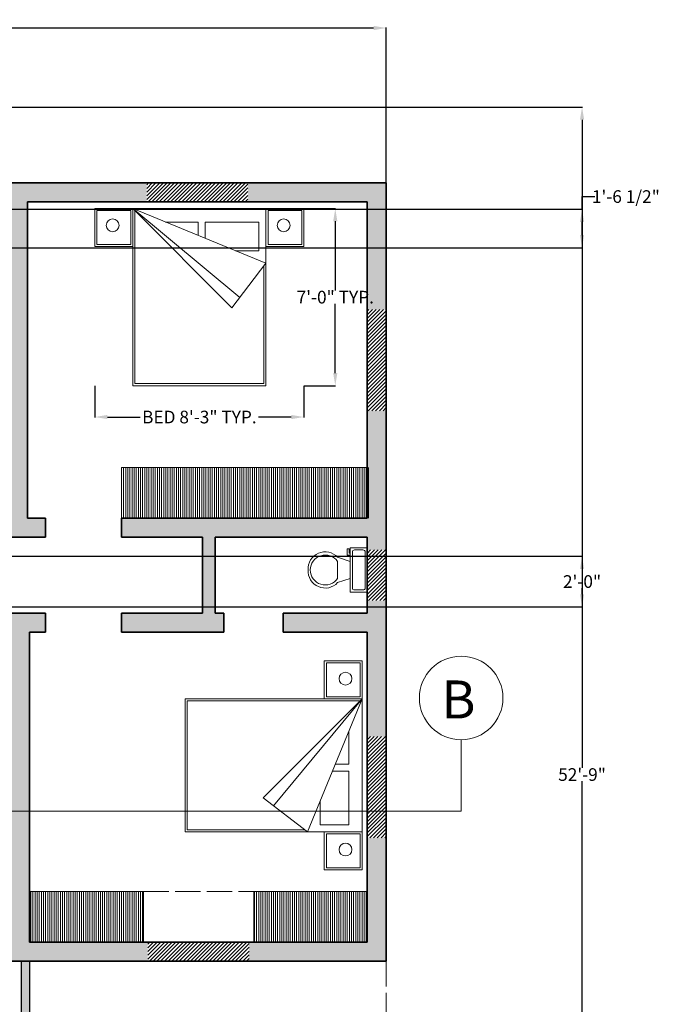
# Model space of a CAD drawing. Units: inches. Extents: x 1966 to 4198, y 2607 to 3884.
# Tile 7 of 8: x 3172 to 3474, y 3411 to 3878. Entities that reach past the tile are written whole.
import ezdxf

# ---------------------------------------------------------------- set-up
doc = ezdxf.new("R2010")
doc.units = ezdxf.units.IN
doc.header["$MEASUREMENT"] = 0
doc.linetypes.add('ACAD_ISO02W100', pattern=[15, 12, -3])
for name, color, linetype, lineweight in [('A-ANNO-SYMB', 90, 'Continuous', 18), ('A-FLOR', 7, 'Continuous', 25), ('A-FLOR-CASE', 163, 'Continuous', 18), ('A-FLOR-CASE-HIDN', 163, 'ACAD_ISO02W100', 13), ('A-FLOR-CASE-PATT', 163, 'Continuous', 13), ('A-FLOR-FIXT', 163, 'Continuous', 18), ('A-GLAZ-PATT', 14, 'Continuous', 13), ('A-WALL', 7, 'Continuous', 35), ('A-WALL-PATT', 252, 'Continuous', 13), ('C-PRKG', 10, 'ACAD_ISO02W100', 18), ('dimension', 90, 'Continuous', 18), ('furniture', 163, 'Continuous', 18)]:
    doc.layers.add(name, color=color, linetype=linetype, lineweight=lineweight)
doc.styles.get("Standard").update_dxf_attribs({"font": 'arial.ttf'})
doc.dimstyles.get("Standard").update_dxf_attribs({"dimtxt": 6, "dimasz": 6, "dimexe": 0.18, "dimexo": 0.0625, "dimgap": 0.09, "dimtad": 0, "dimtih": 1, "dimtoh": 1, "dimdec": 1, "dimzin": 0, "dimdsep": 46, "dimlunit": 3, "dimtxsty": 'Standard', "dimcen": 0.09, "dimadec": 0, "dimazin": 0, "dimtfac": 1, "dimtdec": 1, "dimtofl": 0, "dimtmove": 0, "dimatfit": 3, "dimfxl": 1, "dimtolj": 1, "dimtzin": 0, "dimarcsym": 0})

# ---------------------------------------------------------------- blocks, each defined once
blk = doc.blocks.new('*U14')
for p, q in [((9.5, -6), (9.5, -2)), ((-10, -8.5), (-8, -8.5)), ((-10, -9.5), (-10, -8.5)), ((-8, -8.5), (-8, -8)), ((-7, -8), (-7, -9.5)), ((-4, -8), (-6, -14)), ((4, -8), (6, -14)), ((-7, -9.5), (-10, -9.5)), ((4, -14), (-4, -14))]:
    blk.add_line(p, q)
blk.add_lwpolyline([(10.5, -8), (10.5, 0), (-10.5, 0), (-10.5, -8)], close=True)
for points in [[(-9.5, -2), (-9.5, -6)], [(8.5, -1), (-8.5, -1)], [(-8.5, -7), (8.5, -7)]]:
    blk.add_lwpolyline(points)
for centre, radius, start, end in [((-8.625, -1.875), 0.8839, 81.8699, 188.1301), ((8.625, -1.875), 0.8839, 351.8699, 98.1301), ((-8.625, -6.125), 0.8839, 171.869898, 278.1301), ((8.625, -6.125), 0.8839, 261.8699, 8.1301), ((-0.4772, -19.9188), 8.0953, 133.01722, 273.38), ((0.0374, -19.8731), 7.127, 124.50543, 269.7), ((-0.0373, -19.8731), 7.127, 270.3, 55.4946), ((0.4773, -19.9188), 8.0953, 266.62, 46.9828)]:
    blk.add_arc(centre, radius, start, end)
blk = doc.blocks.new('BED')
at = {"layer": 'furniture'}
for p, q in [((3238.51, 3777.61), (3301.62, 3751.64)), ((3285.43, 3730.55), (3238.51, 3777.61)), ((3238.51, 3777.61), (3289.22, 3735.48)), ((3301.62, 3751.64), (3285.43, 3730.55))]:
    blk.add_line(p, q, dxfattribs=at)
for points in [[(3220.51, 3759.61), (3238.51, 3759.61), (3238.51, 3777.61), (3220.51, 3777.61)], [(3238.51, 3693.61), (3301.62, 3693.61), (3301.62, 3777.61), (3238.51, 3777.61)], [(3301.62, 3759.61), (3319.62, 3759.61), (3319.62, 3777.61), (3301.62, 3777.61)], [(3221.51, 3760.61), (3237.51, 3760.61), (3237.51, 3776.61), (3221.51, 3776.61)], [(3302.62, 3760.61), (3318.62, 3760.61), (3318.62, 3776.61), (3302.62, 3776.61)]]:
    blk.add_lwpolyline(points, close=True, dxfattribs=at)
for points in [[(3239.51, 3776.61), (3239.51, 3694.61), (3300.62, 3694.61), (3300.62, 3750.34)], [(3254.03, 3771.22), (3269.45, 3771.22), (3269.45, 3764.88)], [(3272.78, 3763.51), (3272.78, 3771.22), (3298.23, 3771.22), (3298.23, 3757.59), (3287.16, 3757.59)]]:
    blk.add_lwpolyline(points, dxfattribs=at)
for centre in [(3228.96, 3769.64), (3310.01, 3769.64)]:
    blk.add_circle(centre, 3.03, dxfattribs=at)
blk = doc.blocks.new('PORCH-PARAPET-PLAN')
for p, q in [((0, 86), (0, 0)), ((4, 86), (4, 4)), ((181.42, 86), (181.42, 4)), ((185.42, 86), (185.42, 0)), ((0, 0), (23.64, 0)), ((4, 4), (23.64, 4)), ((23.64, 4), (23.64, 0)), ((83.64, 4), (83.64, 0)), ((83.64, 4), (181.42, 4)), ((83.64, 0), (185.42, 0))]:
    blk.add_line(p, q)
blk = doc.blocks.new('*D51')
at = {"layer": 'Defpoints', "color": 0, "transparency": 16777216}
for p in [(3207.34, 3704.37), (3306.44, 3704.37), (3306.44, 3689.51)]:
    blk.add_point(p, dxfattribs=at)
at = {"layer": 'dimension', "color": 0, "lineweight": -2, "transparency": 16777216}
for p, q in [((3207.34, 3704.31), (3207.34, 3689.33)), ((3306.44, 3704.31), (3306.44, 3689.33)), ((3213.34, 3689.51), (3228.87, 3689.51)), ((3300.44, 3689.51), (3284.92, 3689.51))]:
    blk.add_line(p, q, dxfattribs=at)
at = {"layer": 'dimension', "color": 0, "transparency": 16777216}
for points in [[(3213.34, 3690.51), (3213.34, 3688.51), (3207.34, 3689.51)], [(3300.44, 3690.51), (3300.44, 3688.51), (3306.44, 3689.51)]]:
    blk.add_solid(points, dxfattribs=at)
at = {"layer": 'dimension', "color": 0, "transparency": 16777216, "insert": (3256.89, 3689.51), "char_height": 6, "attachment_point": 5}
blk.add_mtext('\\A1;BED 8\'-3" TYP.', dxfattribs=at)
blk = doc.blocks.new('*D52')
at = {"layer": 'Defpoints', "color": 0, "transparency": 16777216}
for p in [(3306.44, 3788.37), (3321.31, 3788.37), (3306.44, 3704.37)]:
    blk.add_point(p, dxfattribs=at)
at = {"layer": 'dimension', "color": 0, "lineweight": -2, "transparency": 16777216}
for p, q in [((3306.51, 3788.37), (3321.49, 3788.37)), ((3321.31, 3782.37), (3321.31, 3749.53)), ((3321.31, 3710.37), (3321.31, 3743.22)), ((3306.51, 3704.37), (3321.49, 3704.37))]:
    blk.add_line(p, q, dxfattribs=at)
at = {"layer": 'dimension', "color": 0, "transparency": 16777216}
for points in [[(3320.31, 3782.37), (3322.31, 3782.37), (3321.31, 3788.37)], [(3320.31, 3710.37), (3322.31, 3710.37), (3321.31, 3704.37)]]:
    blk.add_solid(points, dxfattribs=at)
at = {"layer": 'dimension', "color": 0, "transparency": 16777216, "insert": (3321.31, 3746.37), "char_height": 6, "attachment_point": 5}
blk.add_mtext('\\A1;7\'-0" TYP.', dxfattribs=at)
blk = doc.blocks.new('*D87')
at = {"layer": 'Defpoints', "color": 0, "transparency": 16777216}
for p in [(3345.44, 3874), (2880.44, 3800.5), (3345.44, 3800.5)]:
    blk.add_point(p, dxfattribs=at)
at = {"layer": 'dimension', "color": 0, "lineweight": -2, "transparency": 16777216}
for p, q in [((2880.44, 3800.57), (2880.44, 3874.18)), ((2886.44, 3874), (3102.55, 3874)), ((3339.44, 3874), (3123.33, 3874)), ((3345.44, 3800.57), (3345.44, 3874.18))]:
    blk.add_line(p, q, dxfattribs=at)
at = {"layer": 'dimension', "color": 0, "transparency": 16777216}
for points in [[(2886.44, 3875), (2886.44, 3873), (2880.44, 3874)], [(3339.44, 3875), (3339.44, 3873), (3345.44, 3874)]]:
    blk.add_solid(points, dxfattribs=at)
at = {"layer": 'dimension', "color": 0, "transparency": 16777216, "insert": (3112.94, 3874), "char_height": 6, "attachment_point": 5}
blk.add_mtext('\\A1;38\'-9"', dxfattribs=at)
blk = doc.blocks.new('*D88')
at = {"layer": 'Defpoints', "color": 0, "transparency": 16777216}
for p in [(3058.44, 3836.5), (3345.44, 3203.44), (3438.28, 3203.44)]:
    blk.add_point(p, dxfattribs=at)
at = {"layer": 'dimension', "color": 0, "lineweight": -2, "transparency": 16777216}
for p, q in [((3058.5, 3836.5), (3438.46, 3836.5)), ((3438.28, 3830.5), (3438.28, 3523.13)), ((3438.28, 3209.44), (3438.28, 3516.82)), ((3345.5, 3203.44), (3438.46, 3203.44))]:
    blk.add_line(p, q, dxfattribs=at)
at = {"layer": 'dimension', "color": 0, "transparency": 16777216}
for points in [[(3437.28, 3830.5), (3439.28, 3830.5), (3438.28, 3836.5)], [(3437.28, 3209.44), (3439.28, 3209.44), (3438.28, 3203.44)]]:
    blk.add_solid(points, dxfattribs=at)
at = {"layer": 'dimension', "color": 0, "transparency": 16777216, "insert": (3438.28, 3519.97), "char_height": 6, "attachment_point": 5}
blk.add_mtext('\\A1;52\'-9"', dxfattribs=at)
blk = doc.blocks.new('*D93')
at = {"layer": 'Defpoints', "color": 0, "transparency": 16777216}
for p in [(2963.74, 3623.5), (3438.28, 3623.5), (2963.74, 3599.5)]:
    blk.add_point(p, dxfattribs=at)
at = {"layer": 'dimension', "color": 0, "lineweight": -2, "transparency": 16777216}
for p, q in [((2963.8, 3623.5), (3438.46, 3623.5)), ((3438.28, 3617.5), (3438.28, 3614.66)), ((3438.28, 3605.5), (3438.28, 3608.35)), ((2963.8, 3599.5), (3438.46, 3599.5))]:
    blk.add_line(p, q, dxfattribs=at)
at = {"layer": 'dimension', "color": 0, "transparency": 16777216}
for points in [[(3437.28, 3617.5), (3439.28, 3617.5), (3438.28, 3623.5)], [(3437.28, 3605.5), (3439.28, 3605.5), (3438.28, 3599.5)]]:
    blk.add_solid(points, dxfattribs=at)
at = {"layer": 'dimension', "color": 0, "transparency": 16777216, "insert": (3438.28, 3611.5), "char_height": 6, "attachment_point": 5}
blk.add_mtext('\\A1;2\'-0"', dxfattribs=at)
blk = doc.blocks.new('*D96')
at = {"layer": 'Defpoints', "color": 0, "transparency": 16777216}
for p in [(2967.99, 3788.06), (3438.28, 3788.06), (2967.99, 3769.8)]:
    blk.add_point(p, dxfattribs=at)
at = {"layer": 'dimension', "color": 0, "lineweight": -2, "transparency": 16777216}
for p, q in [((3438.28, 3788.06), (3438.28, 3794.06)), ((3438.28, 3794.06), (3444.28, 3794.06)), ((2968.06, 3788.06), (3438.46, 3788.06)), ((3438.28, 3775.8), (3438.28, 3782.06)), ((2968.06, 3769.8), (3438.46, 3769.8))]:
    blk.add_line(p, q, dxfattribs=at)
at = {"layer": 'dimension', "color": 0, "transparency": 16777216}
for points in [[(3437.28, 3782.06), (3439.28, 3782.06), (3438.28, 3788.06)], [(3437.28, 3775.8), (3439.28, 3775.8), (3438.28, 3769.8)]]:
    blk.add_solid(points, dxfattribs=at)
at = {"layer": 'dimension', "color": 0, "transparency": 16777216, "insert": (3459.06, 3794.06), "char_height": 6, "attachment_point": 5}
blk.add_mtext('\\A1;1\'-6 1/2"', dxfattribs=at)

msp = doc.modelspace()

# ---------------------------------------------------------------- hatches: boundary and pattern name
at = {"layer": 'A-FLOR-CASE-PATT'}
h = msp.add_hatch(dxfattribs=at)
h.set_pattern_fill('ANSI31', color=256, scale=8, angle=45, style=0)
h.paths.add_polyline_path([(3219.92, 3641.5), (3337.92, 3641.5), (3337.92, 3665.5), (3219.92, 3665.5)])
h = msp.add_hatch(dxfattribs=at)
h.set_pattern_fill('ANSI31', color=256, scale=8, angle=45, style=0)
h.paths.add_polyline_path([(3176.44, 3440.5), (3230.38, 3440.5), (3230.38, 3464.5), (3176.44, 3464.5)])
h = msp.add_hatch(dxfattribs=at)
h.set_pattern_fill('ANSI31', color=256, scale=8, angle=45, style=0)
h.paths.add_polyline_path([(3282.68, 3440.5), (3336.44, 3440.5), (3336.44, 3464.5), (3282.68, 3464.5)])
at = {"layer": 'A-GLAZ-PATT'}
h = msp.add_hatch(dxfattribs=at)
h.set_pattern_fill('ANSI31', color=256, scale=10)
h.set_pattern_definition([(45, (819.9656, 0), (-0.88388348, 0.88388348), [])])
h.paths.add_polyline_path([(2884.94, 3746.62), (2880.44, 3746.62), (2880.44, 3698.62), (2884.94, 3698.62)])
h.paths.add_polyline_path([(2889.44, 3746.62), (2884.94, 3746.62), (2884.94, 3698.62), (2889.44, 3698.62)])
h.paths.add_polyline_path([(2969.44, 3800.5), (2921.44, 3800.5), (2921.44, 3796), (2969.44, 3796)])
h.paths.add_polyline_path([(2969.44, 3796), (2921.44, 3796), (2921.44, 3791.5), (2969.44, 3791.5)])
h.paths.add_polyline_path([(3100.44, 3800.5), (3076.44, 3800.5), (3076.44, 3796), (3100.44, 3796)])
h.paths.add_polyline_path([(3100.44, 3796), (3076.44, 3796), (3076.44, 3791.5), (3100.44, 3791.5)])
h.paths.add_polyline_path([(3154.44, 3800.5), (3130.44, 3800.5), (3130.44, 3796), (3154.44, 3796)])
h.paths.add_polyline_path([(3154.44, 3796), (3130.44, 3796), (3130.44, 3791.5), (3154.44, 3791.5)])
h.paths.add_polyline_path([(3279.94, 3800.5), (3231.94, 3800.5), (3231.94, 3796), (3279.94, 3796)])
h.paths.add_polyline_path([(3279.94, 3796), (3231.94, 3796), (3231.94, 3791.5), (3279.94, 3791.5)])
h.paths.add_polyline_path([(3345.44, 3740.5), (3340.94, 3740.5), (3340.94, 3692.5), (3345.44, 3692.5)])
h.paths.add_polyline_path([(3340.94, 3740.5), (3336.44, 3740.5), (3336.44, 3692.5), (3340.94, 3692.5)])
h.paths.add_polyline_path([(3340.94, 3626.5), (3336.44, 3626.5), (3336.44, 3602.5), (3340.94, 3602.5)])
h.paths.add_polyline_path([(3345.44, 3626.5), (3340.94, 3626.5), (3340.94, 3602.5), (3345.44, 3602.5)])
h.paths.add_polyline_path([(3345.44, 3538), (3340.94, 3538), (3340.94, 3490), (3345.44, 3490)])
h.paths.add_polyline_path([(3340.94, 3538), (3336.44, 3538), (3336.44, 3490), (3340.94, 3490)])
h.paths.add_polyline_path([(3280.44, 3436), (3232.44, 3436), (3232.44, 3431.5), (3280.44, 3431.5)])
h.paths.add_polyline_path([(3280.44, 3440.5), (3232.44, 3440.5), (3232.44, 3436), (3280.44, 3436)])
at = {"layer": 'A-WALL-PATT'}
h = msp.add_hatch(color=256, dxfattribs=at)
h.dxf.hatch_style = 1
h.paths.add_polyline_path([(3010.44, 3599.5), (2889.44, 3599.5), (2889.44, 3698.62), (2880.44, 3698.62), (2880.44, 3590.5), (2880.44, 3539.5), (2889.44, 3539.5), (2889.44, 3590.5), (3010.44, 3590.5)])
h.paths.add_polyline_path([(2889.44, 3491.5), (2880.44, 3491.5), (2880.44, 3431.5), (2924.93, 3431.5), (2924.93, 3440.5), (2889.44, 3440.5)])
h.paths.add_polyline_path([(3008.43, 3440.5), (2972.93, 3440.5), (2972.93, 3431.5), (3008.43, 3431.5)])
h.paths.add_polyline_path([(2995.02, 3431.5), (2991.02, 3431.5), (2991.02, 3345.5), (3014.67, 3345.5), (3014.67, 3349.5), (2995.02, 3349.5)])
h.paths.add_polyline_path([(3232.44, 3440.5), (3176.44, 3440.5), (3176.44, 3587.5), (3183.92, 3587.5), (3183.92, 3591.41), (3183.92, 3596.5), (3167.44, 3596.5), (3167.44, 3440.5), (3092.44, 3440.5), (3092.44, 3590.5), (3083.44, 3590.5), (3083.44, 3440.5), (3056.43, 3440.5), (3056.43, 3438.68), (3056.43, 3431.5), (3092.44, 3431.5), (3232.44, 3431.5)])
h.paths.add_polyline_path([(3176.44, 3431.5), (3172.44, 3431.5), (3172.44, 3349.5), (3074.67, 3349.5), (3074.67, 3345.5), (3176.44, 3345.5)])
h.paths.add_polyline_path([(3345.44, 3490), (3336.44, 3490), (3336.44, 3440.5), (3280.44, 3440.5), (3280.44, 3431.5), (3345.44, 3431.5)])
h.paths.add_polyline_path([(3345.44, 3599.5), (3345.44, 3602.5), (3336.44, 3602.5), (3336.44, 3596.5), (3296.55, 3596.5), (3296.55, 3587.5), (3336.44, 3587.5), (3336.44, 3538), (3345.44, 3538)])
h.paths.add_polyline_path([(3264.44, 3632.5), (3336.44, 3632.5), (3336.44, 3626.5), (3345.44, 3626.5), (3345.44, 3692.5), (3336.44, 3692.5), (3336.44, 3641.5), (3219.92, 3641.5), (3219.92, 3632.5), (3258.44, 3632.5), (3258.44, 3596.5), (3219.95, 3596.5), (3219.95, 3591.41, -0.010779), (3219.92, 3589.86), (3219.92, 3587.5), (3268.55, 3587.5), (3268.55, 3591.7), (3268.55, 3596.5), (3264.44, 3596.5)])
h.paths.add_polyline_path([(3175.44, 3791.5), (3231.94, 3791.5), (3231.94, 3800.5), (3175.44, 3800.5), (3154.44, 3800.5), (3154.44, 3791.5), (3166.44, 3791.5), (3166.44, 3719.5), (3118.44, 3719.5), (3112.44, 3719.5), (3058.44, 3719.5), (3058.44, 3710.5), (3166.44, 3710.5), (3166.44, 3632.5), (3183.92, 3632.5), (3183.92, 3637.87), (3183.92, 3641.5), (3175.44, 3641.5)])
h.paths.add_polyline_path([(3345.44, 3800.5), (3279.94, 3800.5), (3279.94, 3791.5), (3336.44, 3791.5), (3336.44, 3740.5), (3345.44, 3740.5)])
h.paths.add_polyline_path([(3130.44, 3800.5), (3100.44, 3800.5), (3100.44, 3791.5), (3112.44, 3791.5), (3112.44, 3755.5), (3112.44, 3751.71), (3112.44, 3747.5), (3118.44, 3747.5), (3118.44, 3791.5), (3130.44, 3791.5)], flags=17)
h.paths.add_polyline_path([(3076.44, 3800.5), (3058.44, 3800.5), (3058.44, 3796.92), (3058.44, 3791.5), (3058.44, 3749.5), (3084.38, 3749.5), (3084.38, 3751.71, -0.016709), (3084.44, 3753.59), (3084.44, 3755.5), (3064.44, 3755.5), (3064.44, 3791.5), (3076.44, 3791.5)], flags=17)
h.paths.add_polyline_path([(3022.36, 3796.92, -0.017138), (3022.44, 3799.39), (3022.44, 3800.5), (3010.44, 3800.5), (2969.44, 3800.5), (2969.44, 3791.5), (3001.44, 3791.5), (3001.44, 3632.5), (3010.44, 3632.5), (3010.44, 3791.5), (3022.36, 3791.5)])
h.paths.add_polyline_path([(2921.44, 3800.5), (2880.44, 3800.5), (2880.44, 3746.62), (2889.44, 3746.62), (2889.44, 3791.5), (2921.44, 3791.5)])

# ---------------------------------------------------------------- linework, layer by layer
at = {"layer": 'A-ANNO-SYMB'}
for p, q in [((3380.97, 3502.67), (3380.97, 3536.48)), ((2847.64, 3502.67), (3380.97, 3502.67))]:
    msp.add_line(p, q, dxfattribs=at)
msp.add_circle((3380.97, 3556.29), 19.81, dxfattribs=at)
at = {"layer": 'A-FLOR-CASE'}
for p, q in [((3219.92, 3665.5), (3336.44, 3665.5)), ((3219.92, 3665.5), (3219.92, 3641.5)), ((3176.44, 3464.5), (3230.38, 3464.5)), ((3230.38, 3440.5), (3230.38, 3464.5)), ((3282.68, 3440.5), (3282.68, 3464.5)), ((3282.68, 3464.5), (3336.44, 3464.5))]:
    msp.add_line(p, q, dxfattribs=at)
at = {"layer": 'A-FLOR-CASE-HIDN'}
msp.add_line((3230.38, 3464.5), (3282.68, 3464.5), dxfattribs=at)
at = {"layer": 'A-WALL'}
for p, q in [((3175.44, 3800.5), (3058.44, 3800.5)), ((3175.44, 3800.5), (3345.44, 3800.5)), ((3345.44, 3599.5), (3345.44, 3800.5)), ((3175.44, 3641.5), (3175.44, 3791.5)), ((3175.44, 3791.5), (3336.44, 3791.5)), ((3336.44, 3641.5), (3336.44, 3791.5)), ((3175.44, 3641.5), (3183.92, 3641.5)), ((3183.92, 3641.5), (3183.92, 3632.5)), ((3219.92, 3641.5), (3336.44, 3641.5)), ((3219.92, 3641.5), (3219.92, 3632.5)), ((3166.44, 3632.5), (3183.92, 3632.5)), ((3219.92, 3632.5), (3258.44, 3632.5)), ((3258.44, 3632.5), (3258.44, 3596.5)), ((3264.44, 3632.5), (3336.44, 3632.5)), ((3264.44, 3632.5), (3264.44, 3596.5)), ((3336.44, 3632.5), (3336.44, 3596.5)), ((3167.44, 3596.5), (3183.92, 3596.5)), ((3183.92, 3596.5), (3183.92, 3587.5)), ((3219.92, 3596.5), (3258.44, 3596.5)), ((3219.92, 3596.5), (3219.92, 3587.5)), ((3264.44, 3596.5), (3268.55, 3596.5)), ((3268.55, 3596.5), (3268.55, 3587.5)), ((3296.55, 3596.5), (3336.44, 3596.5)), ((3296.55, 3596.5), (3296.55, 3587.5)), ((3345.44, 3599.5), (3345.44, 3431.5)), ((3176.44, 3587.5), (3183.92, 3587.5)), ((3176.44, 3440.5), (3176.44, 3587.5)), ((3219.92, 3587.5), (3268.55, 3587.5)), ((3296.55, 3587.5), (3336.44, 3587.5)), ((3336.44, 3587.5), (3336.44, 3440.5)), ((3176.44, 3440.5), (3336.44, 3440.5)), ((3092.44, 3431.5), (3345.44, 3431.5))]:
    msp.add_line(p, q, dxfattribs=at)
at = {"layer": 'C-PRKG'}
msp.add_line((3345.44, 3431.5), (3345.44, 3203.44), dxfattribs=at)

# ---------------------------------------------------------------- block references
at = {"layer": 'A-FLOR'}
msp.add_blockref('PORCH-PARAPET-PLAN', (2991.02, 3345.5), dxfattribs=at)
at = {"layer": 'A-FLOR-FIXT', "rotation": 270}
msp.add_blockref('*U14', (3336.44, 3616.99), dxfattribs=at)
at = {"layer": 'furniture'}
msp.add_blockref('BED', (-13.18, 10.77), dxfattribs=at)
at = {"layer": 'furniture', "rotation": 270}
msp.add_blockref('BED', (-443.49, 6794.41), dxfattribs=at)

# ---------------------------------------------------------------- texts
at = {"layer": 'A-ANNO-SYMB', "insert": (3371.64, 3564.58), "char_height": 18, "attachment_point": 1}
msp.add_mtext_dynamic_manual_height_columns('B', width=16.3986, gutter_width=1, heights=[0], dxfattribs=at)

# ---------------------------------------------------------------- dimensions: what is measured, and where the dimension line sits
at = {"layer": 'dimension'}
dim = msp.add_linear_dim(base=(3345.44, 3874), p1=(2880.44, 3800.5), p2=(3345.44, 3800.5), dimstyle='Standard', override={"dimdec": 1, "dimlfac": 1, "dimrnd": 0, "dimzin": 1, "dimdsep": 46, "dimlunit": 4, "dimfrac": 2}, dxfattribs=at)
dim.commit()
dim.dimension.update_dxf_attribs({"geometry": '*D87', "text_midpoint": (3112.94, 3874)})
for base, p1, p2, picture, middle in [((3438.28, 3203.44), (3058.44, 3836.5), (3345.44, 3203.44), '*D88', (3438.28, 3519.97)), ((3438.28, 3788.06), (2967.99, 3769.8), (2967.99, 3788.06), '*D96', (3459.06, 3794.06)), ((3438.28, 3623.5), (2963.74, 3599.5), (2963.74, 3623.5), '*D93', (3438.28, 3611.5))]:
    dim = msp.add_linear_dim(base=base, p1=p1, p2=p2, angle=90, dimstyle='Standard', override={"dimdec": 1, "dimlfac": 1, "dimrnd": 0, "dimzin": 1, "dimdsep": 46, "dimlunit": 4, "dimfrac": 2}, dxfattribs=at)
    dim.commit()
    dim.dimension.update_dxf_attribs({"geometry": picture, "text_midpoint": middle})
dim = msp.add_linear_dim(base=(3321.31, 3788.37), p1=(3306.44, 3704.37), p2=(3306.44, 3788.37), angle=90, text='<> TYP.', dimstyle='Standard', override={"dimdec": 1, "dimlfac": 1, "dimrnd": 0, "dimzin": 1, "dimdsep": 46, "dimlunit": 4, "dimfrac": 2}, dxfattribs=at)
dim.commit()
dim.dimension.update_dxf_attribs({"geometry": '*D52', "text_midpoint": (3321.31, 3746.37)})
dim = msp.add_linear_dim(base=(3306.44, 3689.51), p1=(3207.34, 3704.37), p2=(3306.44, 3704.37), text='BED <> TYP.', dimstyle='Standard', override={"dimdec": 1, "dimlfac": 1, "dimrnd": 0, "dimzin": 1, "dimdsep": 46, "dimlunit": 4, "dimfrac": 2}, dxfattribs=at)
dim.commit()
dim.dimension.update_dxf_attribs({"geometry": '*D51', "text_midpoint": (3256.89, 3689.51)})

doc.saveas('drawing.dxf')
